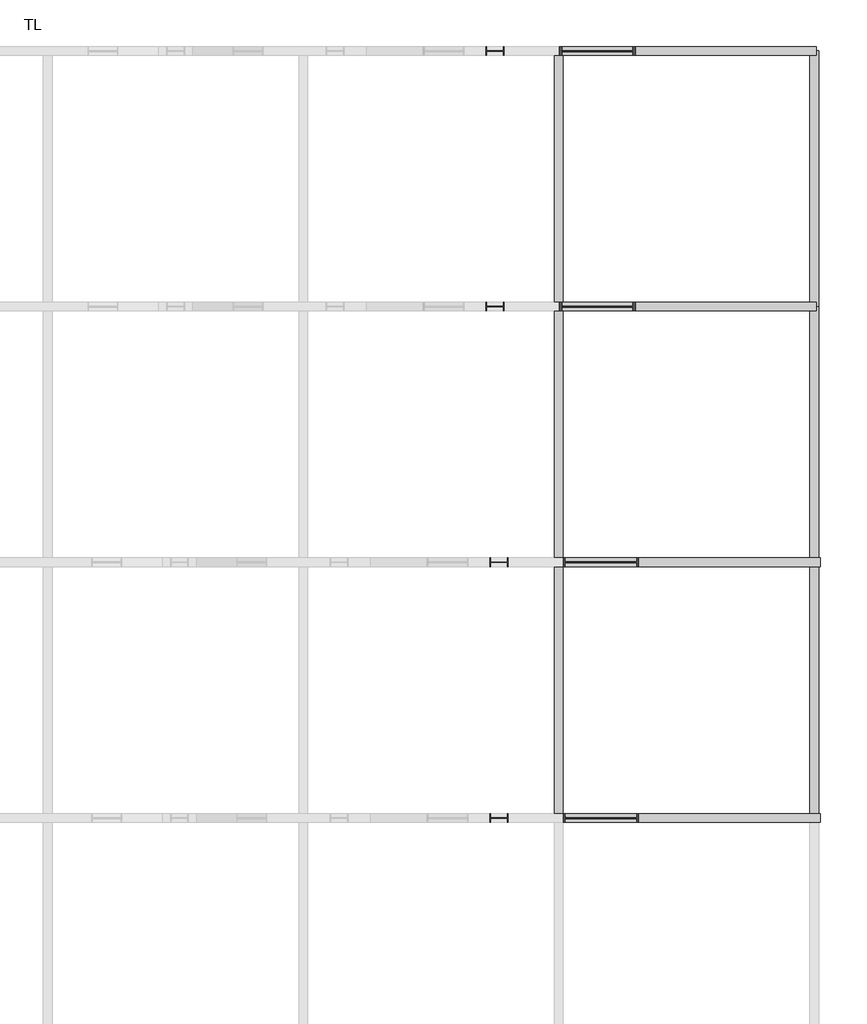
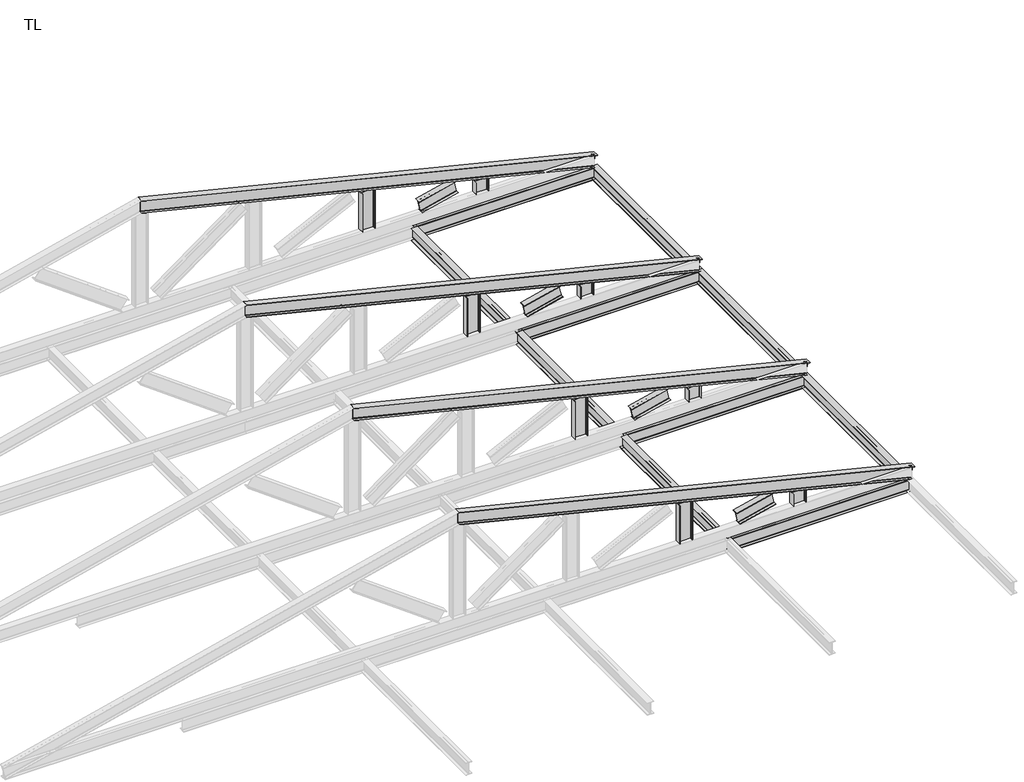
# One storey, part 4 of 4: 26 beams.
"""IFC4 building model written with IfcOpenShell, lengths in millimetres."""

from ifc_helpers import new_model, si_unit, frame, origin, place, context, project, spatial, polyline, circle_curve, ellipse_curve, transform, mapped, element, save
from ifc_brep_helpers import plane_surface, revolved_surface, advanced_brep
from components import w_shapes_w14x30_920474df, w_shapes_w14x30_b44ec7f2, w_shapes_w14x30_809da129, w_shapes_w14x30_95bb247d

model = new_model("IFC4")

# Units and contexts
model_context = context("Model", 3, world=origin())
ifc_project = project(units=[si_unit("LENGTHUNIT", "METRE", prefix="MILLI")], contexts=[model_context])

# Site, building, storey
site = spatial("IfcSite", under=ifc_project)
building = spatial("IfcBuilding", under=site)
storey = spatial("IfcBuildingStorey", under=building, Name="TL", Elevation=8534.4)

# Beams
placement = place(None, origin())
element("IfcBeam", 1, ObjectType="W Shapes : W14X30", at=placement, inside=storey, context=model_context, shape_type="AdvancedBrep", body=[
    advanced_brep(
    [(6535.1598435, 14124.3335479, 8538.7295322), (6535.1598435, 14052.4515479, 8538.7295322), (6537.5667365, 14042.2915479, 8548.6003207), (6611.1574921, 14042.2915479, 8850.3996793), (6613.5643852, 14052.4515479, 8860.2704678), (6613.5643852, 14124.3335479, 8860.2704678), (6615.8810198, 14124.3335479, 8869.7711017), (6615.8810198, 13953.3915479, 8869.7711017), (6613.5643852, 13953.3915479, 8860.2704678), (6613.5643852, 14025.2735479, 8860.2704678), (6611.1574921, 14035.4335479, 8850.3996793), (6537.5667365, 14035.4335479, 8548.6003207), (6535.1598435, 14025.2735479, 8538.7295322), (6535.1598435, 13953.3915479, 8538.7295322), (6532.8432089, 13953.3915479, 8529.2288983), (6532.8432089, 14124.3335479, 8529.2288983), (-5925.6378857, 14124.3335479, 11577.1704505), (-5925.6378857, 14052.4515479, 11577.1704505), (-5925.6378857, 14042.2915479, 11587.6281358), (-5925.6378857, 14042.2915479, 11907.3718642), (-5925.6378857, 14052.4515479, 11917.8295495), (-5925.6378857, 14124.3335479, 11917.8295495), (-5925.6378857, 14124.3335479, 11927.8950717), (-5925.6378857, 13953.3915479, 11927.8950717), (-5925.6378857, 13953.3915479, 11917.8295495), (-5925.6378857, 14025.2735479, 11917.8295495), (-5925.6378857, 14035.4335479, 11907.3718642), (-5925.6378857, 14035.4335479, 11587.6281358), (-5925.6378857, 14025.2735479, 11577.1704505), (-5925.6378857, 13953.3915479, 11577.1704505), (-5925.6378857, 13953.3915479, 11567.1049283), (-5925.6378857, 14124.3335479, 11567.1049283)],
    [
        (0, 1),
        (1, 2, circle_curve(frame((6537.5667365, 14052.4515479, 8548.6003207), z_axis=(-0.971534301878756, 0.0, 0.23689892417011588), x_axis=(0.0, -1.0, 0.0)), 10.16)),
        (2, 3),
        (3, 4, circle_curve(frame((6611.1574921, 14052.4515479, 8850.3996793), z_axis=(-0.971534301878756, 0.0, 0.23689892417011588), x_axis=(0.23689892417011588, 0.0, 0.971534301878756)), 10.16)),
        (4, 5),
        (5, 6),
        (6, 7),
        (7, 8),
        (8, 9),
        (9, 10, circle_curve(frame((6611.1574921, 14025.2735479, 8850.3996793), z_axis=(-0.971534301878756, 0.0, 0.23689892417011588), x_axis=(0.0, 1.0, 0.0)), 10.16)),
        (10, 11),
        (11, 12, circle_curve(frame((6537.5667365, 14025.2735479, 8548.6003207), z_axis=(-0.971534301878756, 0.0, 0.23689892417011588), x_axis=(-0.23689892417011588, 0.0, -0.971534301878756)), 10.16)),
        (12, 13),
        (13, 14),
        (14, 15),
        (15, 0),
        (0, 16),
        (16, 17),
        (17, 1),
        (17, 18, ellipse_curve(frame((-5925.6378857, 14052.4515479, 11587.6281358), z_axis=(-1.0, 0.0, 0.0), x_axis=(0.0, 0.0, 1.0)), 10.4576853, 10.16)),
        (18, 2),
        (18, 19),
        (19, 3),
        (19, 20, ellipse_curve(frame((-5925.6378857, 14052.4515479, 11907.3718642), z_axis=(-1.0, 0.0, 0.0), x_axis=(0.0, 0.0, 1.0)), 10.4576853, 10.16)),
        (20, 4),
        (20, 21),
        (21, 5),
        (21, 22),
        (22, 6),
        (22, 23),
        (23, 7),
        (23, 24),
        (24, 8),
        (24, 25),
        (25, 9),
        (25, 26, ellipse_curve(frame((-5925.6378857, 14025.2735479, 11907.3718642), z_axis=(-1.0, 0.0, 0.0), x_axis=(0.0, 0.0, 1.0)), 10.4576853, 10.16)),
        (26, 10),
        (26, 27),
        (27, 11),
        (27, 28, ellipse_curve(frame((-5925.6378857, 14025.2735479, 11587.6281358), z_axis=(-1.0, 0.0, 0.0), x_axis=(0.0, 0.0, 1.0)), 10.4576853, 10.16)),
        (28, 12),
        (28, 29),
        (29, 13),
        (29, 30),
        (30, 14),
        (30, 31),
        (31, 15),
        (31, 16),
    ],
    [
        plane_surface(frame((6574.3621143, 14038.8625479, 8699.5), z_axis=(0.971534301878756, 0.0, -0.23689892417011588), x_axis=(0.23689892417011588, 0.0, 0.971534301878756))),
        plane_surface(frame((6535.1598435, 14088.3925479, 8538.7295322), z_axis=(0.23689892417011588, 0.0, 0.971534301878756), x_axis=(0.0, -1.0, 0.0))),
        revolved_surface(polyline([(-5928.044778771774, 14042.2915479, 11588.215032583868), (6537.566736564032, 14042.2915479, 8548.600320684385)]), (6537.5667365, 14052.4515479, 8548.6003207), (-0.971534301878756, 0.0, 0.23689892417011588)),
        plane_surface(frame((6574.3621143, 14042.2915479, 8699.5), z_axis=(0.0, 1.0, 0.0), x_axis=(0.23689892417011588, 0.0, 0.971534301878756))),
        revolved_surface(polyline([(-5925.637885691734, 14052.4515479, 11917.82954953391), (6613.564385199924, 14052.4515479, 8860.270467799688)]), (6611.1574921, 14052.4515479, 8850.3996793), (-0.971534301878756, 0.0, 0.23689892417011588)),
        plane_surface(frame((6613.5643852, 14088.3925479, 8860.2704678), z_axis=(-0.23689892417011588, 0.0, -0.971534301878756), x_axis=(0.0, 1.0, 0.0))),
        plane_surface(frame((6614.7227025, 14124.3335479, 8865.0207848), z_axis=(0.0, 1.0, 0.0), x_axis=(0.23689892417011588, 0.0, 0.971534301878756))),
        plane_surface(frame((6615.8810198, 14038.8625479, 8869.7711017), z_axis=(0.23689892417011588, 0.0, 0.971534301878756), x_axis=(0.0, -1.0, 0.0))),
        plane_surface(frame((6614.7227025, 13953.3915479, 8865.0207848), z_axis=(0.0, -1.0, 0.0), x_axis=(-0.23689892417011588, 0.0, -0.971534301878756))),
        plane_surface(frame((6613.5643852, 13989.3325479, 8860.2704678), z_axis=(-0.23689892417011588, 0.0, -0.971534301878756), x_axis=(0.0, 1.0, 0.0))),
        revolved_surface(polyline([(-5928.044778761302, 14035.4335479, 11907.95876102682), (6611.157492130355, 14035.4335479, 8850.3996792926)]), (6611.1574921, 14025.2735479, 8850.3996793), (-0.971534301878756, 0.0, 0.23689892417011588)),
        plane_surface(frame((6574.3621143, 14035.4335479, 8699.5), z_axis=(0.0, -1.0, 0.0), x_axis=(-0.23689892417011588, 0.0, -0.971534301878756))),
        revolved_surface(polyline([(-5930.451671841342, 14025.2735479, 11578.34424407678), (6535.1598434944635, 14025.2735479, 8538.729532177296)]), (6537.5667365, 14025.2735479, 8548.6003207), (-0.971534301878756, 0.0, 0.23689892417011588)),
        plane_surface(frame((6535.1598435, 13989.3325479, 8538.7295322), z_axis=(0.23689892417011588, 0.0, 0.971534301878756), x_axis=(0.0, -1.0, 0.0))),
        plane_surface(frame((6534.0015262, 13953.3915479, 8533.9792152), z_axis=(0.0, -1.0, 0.0), x_axis=(-0.23689892417011588, 0.0, -0.971534301878756))),
        plane_surface(frame((6532.8432089, 14038.8625479, 8529.2288983), z_axis=(-0.23689892417011588, 0.0, -0.971534301878756), x_axis=(0.0, 1.0, 0.0))),
        plane_surface(frame((6534.0015262, 14124.3335479, 8533.9792152), z_axis=(0.0, 1.0, 0.0), x_axis=(0.23689892417011588, 0.0, 0.971534301878756))),
        plane_surface(frame((-5925.6378857, 14038.8625479, 11927.8950717), z_axis=(-1.0, 0.0, 0.0), x_axis=(0.0, 1.0, 0.0))),
    ],
    [
        (0, [[1, 2, 3, 4, 5, 6, 7, 8, 9, 10, 11, 12, 13, 14, 15, 16]]),
        (1, [[-1, 17, 18, 19]]),
        (2, [[-2, -19, 20, 21]]),
        (3, [[-3, -21, 22, 23]]),
        (4, [[-4, -23, 24, 25]]),
        (5, [[-5, -25, 26, 27]]),
        (6, [[-6, -27, 28, 29]]),
        (7, [[-7, -29, 30, 31]]),
        (8, [[-8, -31, 32, 33]]),
        (9, [[-9, -33, 34, 35]]),
        (10, [[-10, -35, 36, 37]]),
        (11, [[-11, -37, 38, 39]]),
        (12, [[-12, -39, 40, 41]]),
        (13, [[-13, -41, 42, 43]]),
        (14, [[-14, -43, 44, 45]]),
        (15, [[-15, -45, 46, 47]]),
        (16, [[-16, -47, 48, -17]]),
        (17, [[-48, -46, -44, -42, -40, -38, -36, -34, -32, -30, -28, -26, -24, -22, -20, -18]]),
    ],
),
])
element("IfcBeam", 2, ObjectType="W Shapes : W14X30", at=placement, inside=storey, context=model_context, shape_type="AdvancedBrep", body=[
    advanced_brep(
    [(6611.3598435, 9124.3335479, 8538.7295322), (6611.3598435, 9052.4515479, 8538.7295322), (6613.7667365, 9042.2915479, 8548.6003207), (6687.3574921, 9042.2915479, 8850.3996793), (6689.7643852, 9052.4515479, 8860.2704678), (6689.7643852, 9124.3335479, 8860.2704678), (6692.0810198, 9124.3335479, 8869.7711017), (6692.0810198, 8953.3915479, 8869.7711017), (6689.7643852, 8953.3915479, 8860.2704678), (6689.7643852, 9025.2735479, 8860.2704678), (6687.3574921, 9035.4335479, 8850.3996793), (6613.7667365, 9035.4335479, 8548.6003207), (6611.3598435, 9025.2735479, 8538.7295322), (6611.3598435, 8953.3915479, 8538.7295322), (6609.0432089, 8953.3915479, 8529.2288983), (6609.0432089, 9124.3335479, 8529.2288983), (-5849.4378857, 9124.3335479, 11577.1704505), (-5849.4378857, 9052.4515479, 11577.1704505), (-5849.4378857, 9042.2915479, 11587.6281358), (-5849.4378857, 9042.2915479, 11907.3718642), (-5849.4378857, 9052.4515479, 11917.8295495), (-5849.4378857, 9124.3335479, 11917.8295495), (-5849.4378857, 9124.3335479, 11927.8950717), (-5849.4378857, 8953.3915479, 11927.8950717), (-5849.4378857, 8953.3915479, 11917.8295495), (-5849.4378857, 9025.2735479, 11917.8295495), (-5849.4378857, 9035.4335479, 11907.3718642), (-5849.4378857, 9035.4335479, 11587.6281358), (-5849.4378857, 9025.2735479, 11577.1704505), (-5849.4378857, 8953.3915479, 11577.1704505), (-5849.4378857, 8953.3915479, 11567.1049283), (-5849.4378857, 9124.3335479, 11567.1049283)],
    [
        (0, 1),
        (1, 2, circle_curve(frame((6613.7667365, 9052.4515479, 8548.6003207), z_axis=(-0.971534301878756, 0.0, 0.23689892417011588), x_axis=(0.0, -1.0, 0.0)), 10.16)),
        (2, 3),
        (3, 4, circle_curve(frame((6687.3574921, 9052.4515479, 8850.3996793), z_axis=(-0.971534301878756, 0.0, 0.23689892417011588), x_axis=(0.23689892417011588, 0.0, 0.971534301878756)), 10.16)),
        (4, 5),
        (5, 6),
        (6, 7),
        (7, 8),
        (8, 9),
        (9, 10, circle_curve(frame((6687.3574921, 9025.2735479, 8850.3996793), z_axis=(-0.971534301878756, 0.0, 0.23689892417011588), x_axis=(0.0, 1.0, 0.0)), 10.16)),
        (10, 11),
        (11, 12, circle_curve(frame((6613.7667365, 9025.2735479, 8548.6003207), z_axis=(-0.971534301878756, 0.0, 0.23689892417011588), x_axis=(-0.23689892417011588, 0.0, -0.971534301878756)), 10.16)),
        (12, 13),
        (13, 14),
        (14, 15),
        (15, 0),
        (0, 16),
        (16, 17),
        (17, 1),
        (17, 18, ellipse_curve(frame((-5849.4378857, 9052.4515479, 11587.6281358), z_axis=(-1.0, 0.0, 0.0), x_axis=(0.0, 0.0, 1.0)), 10.4576853, 10.16)),
        (18, 2),
        (18, 19),
        (19, 3),
        (19, 20, ellipse_curve(frame((-5849.4378857, 9052.4515479, 11907.3718642), z_axis=(-1.0, 0.0, 0.0), x_axis=(0.0, 0.0, 1.0)), 10.4576853, 10.16)),
        (20, 4),
        (20, 21),
        (21, 5),
        (21, 22),
        (22, 6),
        (22, 23),
        (23, 7),
        (23, 24),
        (24, 8),
        (24, 25),
        (25, 9),
        (25, 26, ellipse_curve(frame((-5849.4378857, 9025.2735479, 11907.3718642), z_axis=(-1.0, 0.0, 0.0), x_axis=(0.0, 0.0, 1.0)), 10.4576853, 10.16)),
        (26, 10),
        (26, 27),
        (27, 11),
        (27, 28, ellipse_curve(frame((-5849.4378857, 9025.2735479, 11587.6281358), z_axis=(-1.0, 0.0, 0.0), x_axis=(0.0, 0.0, 1.0)), 10.4576853, 10.16)),
        (28, 12),
        (28, 29),
        (29, 13),
        (29, 30),
        (30, 14),
        (30, 31),
        (31, 15),
        (31, 16),
    ],
    [
        plane_surface(frame((6650.5621143, 9038.8625479, 8699.5), z_axis=(0.971534301878756, 0.0, -0.23689892417011588), x_axis=(0.23689892417011588, 0.0, 0.971534301878756))),
        plane_surface(frame((6611.3598435, 9088.3925479, 8538.7295322), z_axis=(0.23689892417011588, 0.0, 0.971534301878756), x_axis=(0.0, -1.0, 0.0))),
        revolved_surface(polyline([(-5851.844778771774, 9042.2915479, 11588.215032583868), (6613.766736564033, 9042.2915479, 8548.600320684385)]), (6613.7667365, 9052.4515479, 8548.6003207), (-0.971534301878756, 0.0, 0.23689892417011588)),
        plane_surface(frame((6650.5621143, 9042.2915479, 8699.5), z_axis=(0.0, 1.0, 0.0), x_axis=(0.23689892417011588, 0.0, 0.971534301878756))),
        revolved_surface(polyline([(-5849.437885691734, 9052.4515479, 11917.82954953391), (6689.764385199924, 9052.4515479, 8860.270467799688)]), (6687.3574921, 9052.4515479, 8850.3996793), (-0.971534301878756, 0.0, 0.23689892417011588)),
        plane_surface(frame((6689.7643852, 9088.3925479, 8860.2704678), z_axis=(-0.23689892417011588, 0.0, -0.971534301878756), x_axis=(0.0, 1.0, 0.0))),
        plane_surface(frame((6690.9227025, 9124.3335479, 8865.0207848), z_axis=(0.0, 1.0, 0.0), x_axis=(0.23689892417011588, 0.0, 0.971534301878756))),
        plane_surface(frame((6692.0810198, 9038.8625479, 8869.7711017), z_axis=(0.23689892417011588, 0.0, 0.971534301878756), x_axis=(0.0, -1.0, 0.0))),
        plane_surface(frame((6690.9227025, 8953.3915479, 8865.0207848), z_axis=(0.0, -1.0, 0.0), x_axis=(-0.23689892417011588, 0.0, -0.971534301878756))),
        plane_surface(frame((6689.7643852, 8989.3325479, 8860.2704678), z_axis=(-0.23689892417011588, 0.0, -0.971534301878756), x_axis=(0.0, 1.0, 0.0))),
        revolved_surface(polyline([(-5851.844778761302, 9035.4335479, 11907.95876102682), (6687.357492130355, 9035.4335479, 8850.3996792926)]), (6687.3574921, 9025.2735479, 8850.3996793), (-0.971534301878756, 0.0, 0.23689892417011588)),
        plane_surface(frame((6650.5621143, 9035.4335479, 8699.5), z_axis=(0.0, -1.0, 0.0), x_axis=(-0.23689892417011588, 0.0, -0.971534301878756))),
        revolved_surface(polyline([(-5854.251671841343, 9025.2735479, 11578.34424407678), (6611.359843494464, 9025.2735479, 8538.729532177296)]), (6613.7667365, 9025.2735479, 8548.6003207), (-0.971534301878756, 0.0, 0.23689892417011588)),
        plane_surface(frame((6611.3598435, 8989.3325479, 8538.7295322), z_axis=(0.23689892417011588, 0.0, 0.971534301878756), x_axis=(0.0, -1.0, 0.0))),
        plane_surface(frame((6610.2015262, 8953.3915479, 8533.9792152), z_axis=(0.0, -1.0, 0.0), x_axis=(-0.23689892417011588, 0.0, -0.971534301878756))),
        plane_surface(frame((6609.0432089, 9038.8625479, 8529.2288983), z_axis=(-0.23689892417011588, 0.0, -0.971534301878756), x_axis=(0.0, 1.0, 0.0))),
        plane_surface(frame((6610.2015262, 9124.3335479, 8533.9792152), z_axis=(0.0, 1.0, 0.0), x_axis=(0.23689892417011588, 0.0, 0.971534301878756))),
        plane_surface(frame((-5849.4378857, 9038.8625479, 11927.8950717), z_axis=(-1.0, 0.0, 0.0), x_axis=(0.0, 1.0, 0.0))),
    ],
    [
        (0, [[1, 2, 3, 4, 5, 6, 7, 8, 9, 10, 11, 12, 13, 14, 15, 16]]),
        (1, [[-1, 17, 18, 19]]),
        (2, [[-2, -19, 20, 21]]),
        (3, [[-3, -21, 22, 23]]),
        (4, [[-4, -23, 24, 25]]),
        (5, [[-5, -25, 26, 27]]),
        (6, [[-6, -27, 28, 29]]),
        (7, [[-7, -29, 30, 31]]),
        (8, [[-8, -31, 32, 33]]),
        (9, [[-9, -33, 34, 35]]),
        (10, [[-10, -35, 36, 37]]),
        (11, [[-11, -37, 38, 39]]),
        (12, [[-12, -39, 40, 41]]),
        (13, [[-13, -41, 42, 43]]),
        (14, [[-14, -43, 44, 45]]),
        (15, [[-15, -45, 46, 47]]),
        (16, [[-16, -47, 48, -17]]),
        (17, [[-48, -46, -44, -42, -40, -38, -36, -34, -32, -30, -28, -26, -24, -22, -20, -18]]),
    ],
),
])
element("IfcBeam", 3, ObjectType="W Shapes : W14X30", at=placement, inside=storey, context=model_context, shape_type="AdvancedBrep", body=[
    advanced_brep(
    [(6611.3598435, 4124.3335479, 8538.7295322), (6611.3598435, 4052.4515479, 8538.7295322), (6613.7667365, 4042.2915479, 8548.6003207), (6687.3574921, 4042.2915479, 8850.3996793), (6689.7643852, 4052.4515479, 8860.2704678), (6689.7643852, 4124.3335479, 8860.2704678), (6692.0810198, 4124.3335479, 8869.7711017), (6692.0810198, 3953.3915479, 8869.7711017), (6689.7643852, 3953.3915479, 8860.2704678), (6689.7643852, 4025.2735479, 8860.2704678), (6687.3574921, 4035.4335479, 8850.3996793), (6613.7667365, 4035.4335479, 8548.6003207), (6611.3598435, 4025.2735479, 8538.7295322), (6611.3598435, 3953.3915479, 8538.7295322), (6609.0432089, 3953.3915479, 8529.2288983), (6609.0432089, 4124.3335479, 8529.2288983), (-5849.4378857, 4124.3335479, 11577.1704505), (-5849.4378857, 4052.4515479, 11577.1704505), (-5849.4378857, 4042.2915479, 11587.6281358), (-5849.4378857, 4042.2915479, 11907.3718642), (-5849.4378857, 4052.4515479, 11917.8295495), (-5849.4378857, 4124.3335479, 11917.8295495), (-5849.4378857, 4124.3335479, 11927.8950717), (-5849.4378857, 3953.3915479, 11927.8950717), (-5849.4378857, 3953.3915479, 11917.8295495), (-5849.4378857, 4025.2735479, 11917.8295495), (-5849.4378857, 4035.4335479, 11907.3718642), (-5849.4378857, 4035.4335479, 11587.6281358), (-5849.4378857, 4025.2735479, 11577.1704505), (-5849.4378857, 3953.3915479, 11577.1704505), (-5849.4378857, 3953.3915479, 11567.1049283), (-5849.4378857, 4124.3335479, 11567.1049283)],
    [
        (0, 1),
        (1, 2, circle_curve(frame((6613.7667365, 4052.4515479, 8548.6003207), z_axis=(-0.971534301878756, 0.0, 0.23689892417011588), x_axis=(0.0, -1.0, 0.0)), 10.16)),
        (2, 3),
        (3, 4, circle_curve(frame((6687.3574921, 4052.4515479, 8850.3996793), z_axis=(-0.971534301878756, 0.0, 0.23689892417011588), x_axis=(0.23689892417011588, 0.0, 0.971534301878756)), 10.16)),
        (4, 5),
        (5, 6),
        (6, 7),
        (7, 8),
        (8, 9),
        (9, 10, circle_curve(frame((6687.3574921, 4025.2735479, 8850.3996793), z_axis=(-0.971534301878756, 0.0, 0.23689892417011588), x_axis=(0.0, 1.0, 0.0)), 10.16)),
        (10, 11),
        (11, 12, circle_curve(frame((6613.7667365, 4025.2735479, 8548.6003207), z_axis=(-0.971534301878756, 0.0, 0.23689892417011588), x_axis=(-0.23689892417011588, 0.0, -0.971534301878756)), 10.16)),
        (12, 13),
        (13, 14),
        (14, 15),
        (15, 0),
        (0, 16),
        (16, 17),
        (17, 1),
        (17, 18, ellipse_curve(frame((-5849.4378857, 4052.4515479, 11587.6281358), z_axis=(-1.0, 0.0, 0.0), x_axis=(0.0, 0.0, 1.0)), 10.4576853, 10.16)),
        (18, 2),
        (18, 19),
        (19, 3),
        (19, 20, ellipse_curve(frame((-5849.4378857, 4052.4515479, 11907.3718642), z_axis=(-1.0, 0.0, 0.0), x_axis=(0.0, 0.0, 1.0)), 10.4576853, 10.16)),
        (20, 4),
        (20, 21),
        (21, 5),
        (21, 22),
        (22, 6),
        (22, 23),
        (23, 7),
        (23, 24),
        (24, 8),
        (24, 25),
        (25, 9),
        (25, 26, ellipse_curve(frame((-5849.4378857, 4025.2735479, 11907.3718642), z_axis=(-1.0, 0.0, 0.0), x_axis=(0.0, 0.0, 1.0)), 10.4576853, 10.16)),
        (26, 10),
        (26, 27),
        (27, 11),
        (27, 28, ellipse_curve(frame((-5849.4378857, 4025.2735479, 11587.6281358), z_axis=(-1.0, 0.0, 0.0), x_axis=(0.0, 0.0, 1.0)), 10.4576853, 10.16)),
        (28, 12),
        (28, 29),
        (29, 13),
        (29, 30),
        (30, 14),
        (30, 31),
        (31, 15),
        (31, 16),
    ],
    [
        plane_surface(frame((6650.5621143, 4038.8625479, 8699.5), z_axis=(0.971534301878756, 0.0, -0.23689892417011588), x_axis=(0.23689892417011588, 0.0, 0.971534301878756))),
        plane_surface(frame((6611.3598435, 4088.3925479, 8538.7295322), z_axis=(0.23689892417011588, 0.0, 0.971534301878756), x_axis=(0.0, -1.0, 0.0))),
        revolved_surface(polyline([(-5851.844778771774, 4042.2915479000003, 11588.215032583868), (6613.766736564033, 4042.2915479000003, 8548.600320684385)]), (6613.7667365, 4052.4515479, 8548.6003207), (-0.971534301878756, 0.0, 0.23689892417011588)),
        plane_surface(frame((6650.5621143, 4042.2915479, 8699.5), z_axis=(0.0, 1.0, 0.0), x_axis=(0.23689892417011588, 0.0, 0.971534301878756))),
        revolved_surface(polyline([(-5849.437885691734, 4052.4515479, 11917.82954953391), (6689.764385199924, 4052.4515479, 8860.270467799688)]), (6687.3574921, 4052.4515479, 8850.3996793), (-0.971534301878756, 0.0, 0.23689892417011588)),
        plane_surface(frame((6689.7643852, 4088.3925479, 8860.2704678), z_axis=(-0.23689892417011588, 0.0, -0.971534301878756), x_axis=(0.0, 1.0, 0.0))),
        plane_surface(frame((6690.9227025, 4124.3335479, 8865.0207848), z_axis=(0.0, 1.0, 0.0), x_axis=(0.23689892417011588, 0.0, 0.971534301878756))),
        plane_surface(frame((6692.0810198, 4038.8625479, 8869.7711017), z_axis=(0.23689892417011588, 0.0, 0.971534301878756), x_axis=(0.0, -1.0, 0.0))),
        plane_surface(frame((6690.9227025, 3953.3915479, 8865.0207848), z_axis=(0.0, -1.0, 0.0), x_axis=(-0.23689892417011588, 0.0, -0.971534301878756))),
        plane_surface(frame((6689.7643852, 3989.3325479, 8860.2704678), z_axis=(-0.23689892417011588, 0.0, -0.971534301878756), x_axis=(0.0, 1.0, 0.0))),
        revolved_surface(polyline([(-5851.844778761302, 4035.4335478999997, 11907.95876102682), (6687.357492130355, 4035.4335478999997, 8850.3996792926)]), (6687.3574921, 4025.2735479, 8850.3996793), (-0.971534301878756, 0.0, 0.23689892417011588)),
        plane_surface(frame((6650.5621143, 4035.4335479, 8699.5), z_axis=(0.0, -1.0, 0.0), x_axis=(-0.23689892417011588, 0.0, -0.971534301878756))),
        revolved_surface(polyline([(-5854.251671841343, 4025.2735479, 11578.34424407678), (6611.359843494464, 4025.2735479, 8538.729532177296)]), (6613.7667365, 4025.2735479, 8548.6003207), (-0.971534301878756, 0.0, 0.23689892417011588)),
        plane_surface(frame((6611.3598435, 3989.3325479, 8538.7295322), z_axis=(0.23689892417011588, 0.0, 0.971534301878756), x_axis=(0.0, -1.0, 0.0))),
        plane_surface(frame((6610.2015262, 3953.3915479, 8533.9792152), z_axis=(0.0, -1.0, 0.0), x_axis=(-0.23689892417011588, 0.0, -0.971534301878756))),
        plane_surface(frame((6609.0432089, 4038.8625479, 8529.2288983), z_axis=(-0.23689892417011588, 0.0, -0.971534301878756), x_axis=(0.0, 1.0, 0.0))),
        plane_surface(frame((6610.2015262, 4124.3335479, 8533.9792152), z_axis=(0.0, 1.0, 0.0), x_axis=(0.23689892417011588, 0.0, 0.971534301878756))),
        plane_surface(frame((-5849.4378857, 4038.8625479, 11927.8950717), z_axis=(-1.0, 0.0, 0.0), x_axis=(0.0, 1.0, 0.0))),
    ],
    [
        (0, [[1, 2, 3, 4, 5, 6, 7, 8, 9, 10, 11, 12, 13, 14, 15, 16]]),
        (1, [[-1, 17, 18, 19]]),
        (2, [[-2, -19, 20, 21]]),
        (3, [[-3, -21, 22, 23]]),
        (4, [[-4, -23, 24, 25]]),
        (5, [[-5, -25, 26, 27]]),
        (6, [[-6, -27, 28, 29]]),
        (7, [[-7, -29, 30, 31]]),
        (8, [[-8, -31, 32, 33]]),
        (9, [[-9, -33, 34, 35]]),
        (10, [[-10, -35, 36, 37]]),
        (11, [[-11, -37, 38, 39]]),
        (12, [[-12, -39, 40, 41]]),
        (13, [[-13, -41, 42, 43]]),
        (14, [[-14, -43, 44, 45]]),
        (15, [[-15, -45, 46, 47]]),
        (16, [[-16, -47, 48, -17]]),
        (17, [[-48, -46, -44, -42, -40, -38, -36, -34, -32, -30, -28, -26, -24, -22, -20, -18]]),
    ],
),
])
element("IfcBeam", 4, ObjectType="W Shapes : W14X30", at=placement, inside=storey, context=model_context, shape_type="AdvancedBrep", body=[
    advanced_brep(
    [(6535.1598435, 19124.3335479, 8538.7295322), (6535.1598435, 19052.4515479, 8538.7295322), (6537.5667365, 19042.2915479, 8548.6003207), (6611.1574921, 19042.2915479, 8850.3996793), (6613.5643852, 19052.4515479, 8860.2704678), (6613.5643852, 19124.3335479, 8860.2704678), (6615.8810198, 19124.3335479, 8869.7711017), (6615.8810198, 18953.3915479, 8869.7711017), (6613.5643852, 18953.3915479, 8860.2704678), (6613.5643852, 19025.2735479, 8860.2704678), (6611.1574921, 19035.4335479, 8850.3996793), (6537.5667365, 19035.4335479, 8548.6003207), (6535.1598435, 19025.2735479, 8538.7295322), (6535.1598435, 18953.3915479, 8538.7295322), (6532.8432089, 18953.3915479, 8529.2288983), (6532.8432089, 19124.3335479, 8529.2288983), (-5925.6378857, 19124.3335479, 11577.1704505), (-5925.6378857, 19052.4515479, 11577.1704505), (-5925.6378857, 19042.2915479, 11587.6281358), (-5925.6378857, 19042.2915479, 11907.3718642), (-5925.6378857, 19052.4515479, 11917.8295495), (-5925.6378857, 19124.3335479, 11917.8295495), (-5925.6378857, 19124.3335479, 11927.8950717), (-5925.6378857, 18953.3915479, 11927.8950717), (-5925.6378857, 18953.3915479, 11917.8295495), (-5925.6378857, 19025.2735479, 11917.8295495), (-5925.6378857, 19035.4335479, 11907.3718642), (-5925.6378857, 19035.4335479, 11587.6281358), (-5925.6378857, 19025.2735479, 11577.1704505), (-5925.6378857, 18953.3915479, 11577.1704505), (-5925.6378857, 18953.3915479, 11567.1049283), (-5925.6378857, 19124.3335479, 11567.1049283)],
    [
        (0, 1),
        (1, 2, circle_curve(frame((6537.5667365, 19052.4515479, 8548.6003207), z_axis=(-0.971534301878756, 0.0, 0.23689892417011588), x_axis=(0.0, -1.0, 0.0)), 10.16)),
        (2, 3),
        (3, 4, circle_curve(frame((6611.1574921, 19052.4515479, 8850.3996793), z_axis=(-0.971534301878756, 0.0, 0.23689892417011588), x_axis=(0.23689892417011588, 0.0, 0.971534301878756)), 10.16)),
        (4, 5),
        (5, 6),
        (6, 7),
        (7, 8),
        (8, 9),
        (9, 10, circle_curve(frame((6611.1574921, 19025.2735479, 8850.3996793), z_axis=(-0.971534301878756, 0.0, 0.23689892417011588), x_axis=(0.0, 1.0, 0.0)), 10.16)),
        (10, 11),
        (11, 12, circle_curve(frame((6537.5667365, 19025.2735479, 8548.6003207), z_axis=(-0.971534301878756, 0.0, 0.23689892417011588), x_axis=(-0.23689892417011588, 0.0, -0.971534301878756)), 10.16)),
        (12, 13),
        (13, 14),
        (14, 15),
        (15, 0),
        (0, 16),
        (16, 17),
        (17, 1),
        (17, 18, ellipse_curve(frame((-5925.6378857, 19052.4515479, 11587.6281358), z_axis=(-1.0, 0.0, 0.0), x_axis=(0.0, 0.0, 1.0)), 10.4576853, 10.16)),
        (18, 2),
        (18, 19),
        (19, 3),
        (19, 20, ellipse_curve(frame((-5925.6378857, 19052.4515479, 11907.3718642), z_axis=(-1.0, 0.0, 0.0), x_axis=(0.0, 0.0, 1.0)), 10.4576853, 10.16)),
        (20, 4),
        (20, 21),
        (21, 5),
        (21, 22),
        (22, 6),
        (22, 23),
        (23, 7),
        (23, 24),
        (24, 8),
        (24, 25),
        (25, 9),
        (25, 26, ellipse_curve(frame((-5925.6378857, 19025.2735479, 11907.3718642), z_axis=(-1.0, 0.0, 0.0), x_axis=(0.0, 0.0, 1.0)), 10.4576853, 10.16)),
        (26, 10),
        (26, 27),
        (27, 11),
        (27, 28, ellipse_curve(frame((-5925.6378857, 19025.2735479, 11587.6281358), z_axis=(-1.0, 0.0, 0.0), x_axis=(0.0, 0.0, 1.0)), 10.4576853, 10.16)),
        (28, 12),
        (28, 29),
        (29, 13),
        (29, 30),
        (30, 14),
        (30, 31),
        (31, 15),
        (31, 16),
    ],
    [
        plane_surface(frame((6574.3621143, 19038.8625479, 8699.5), z_axis=(0.971534301878756, 0.0, -0.23689892417011588), x_axis=(0.23689892417011588, 0.0, 0.971534301878756))),
        plane_surface(frame((6535.1598435, 19088.3925479, 8538.7295322), z_axis=(0.23689892417011588, 0.0, 0.971534301878756), x_axis=(0.0, -1.0, 0.0))),
        revolved_surface(polyline([(-5928.044778771774, 19042.2915479, 11588.215032583868), (6537.566736564032, 19042.2915479, 8548.600320684385)]), (6537.5667365, 19052.4515479, 8548.6003207), (-0.971534301878756, 0.0, 0.23689892417011588)),
        plane_surface(frame((6574.3621143, 19042.2915479, 8699.5), z_axis=(0.0, 1.0, 0.0), x_axis=(0.23689892417011588, 0.0, 0.971534301878756))),
        revolved_surface(polyline([(-5925.637885691734, 19052.4515479, 11917.82954953391), (6613.564385199924, 19052.4515479, 8860.270467799688)]), (6611.1574921, 19052.4515479, 8850.3996793), (-0.971534301878756, 0.0, 0.23689892417011588)),
        plane_surface(frame((6613.5643852, 19088.3925479, 8860.2704678), z_axis=(-0.23689892417011588, 0.0, -0.971534301878756), x_axis=(0.0, 1.0, 0.0))),
        plane_surface(frame((6614.7227025, 19124.3335479, 8865.0207848), z_axis=(0.0, 1.0, 0.0), x_axis=(0.23689892417011588, 0.0, 0.971534301878756))),
        plane_surface(frame((6615.8810198, 19038.8625479, 8869.7711017), z_axis=(0.23689892417011588, 0.0, 0.971534301878756), x_axis=(0.0, -1.0, 0.0))),
        plane_surface(frame((6614.7227025, 18953.3915479, 8865.0207848), z_axis=(0.0, -1.0, 0.0), x_axis=(-0.23689892417011588, 0.0, -0.971534301878756))),
        plane_surface(frame((6613.5643852, 18989.3325479, 8860.2704678), z_axis=(-0.23689892417011588, 0.0, -0.971534301878756), x_axis=(0.0, 1.0, 0.0))),
        revolved_surface(polyline([(-5928.044778761302, 19035.4335479, 11907.95876102682), (6611.157492130355, 19035.4335479, 8850.3996792926)]), (6611.1574921, 19025.2735479, 8850.3996793), (-0.971534301878756, 0.0, 0.23689892417011588)),
        plane_surface(frame((6574.3621143, 19035.4335479, 8699.5), z_axis=(0.0, -1.0, 0.0), x_axis=(-0.23689892417011588, 0.0, -0.971534301878756))),
        revolved_surface(polyline([(-5930.451671841342, 19025.2735479, 11578.34424407678), (6535.1598434944635, 19025.2735479, 8538.729532177296)]), (6537.5667365, 19025.2735479, 8548.6003207), (-0.971534301878756, 0.0, 0.23689892417011588)),
        plane_surface(frame((6535.1598435, 18989.3325479, 8538.7295322), z_axis=(0.23689892417011588, 0.0, 0.971534301878756), x_axis=(0.0, -1.0, 0.0))),
        plane_surface(frame((6534.0015262, 18953.3915479, 8533.9792152), z_axis=(0.0, -1.0, 0.0), x_axis=(-0.23689892417011588, 0.0, -0.971534301878756))),
        plane_surface(frame((6532.8432089, 19038.8625479, 8529.2288983), z_axis=(-0.23689892417011588, 0.0, -0.971534301878756), x_axis=(0.0, 1.0, 0.0))),
        plane_surface(frame((6534.0015262, 19124.3335479, 8533.9792152), z_axis=(0.0, 1.0, 0.0), x_axis=(0.23689892417011588, 0.0, 0.971534301878756))),
        plane_surface(frame((-5925.6378857, 19038.8625479, 11927.8950717), z_axis=(-1.0, 0.0, 0.0), x_axis=(0.0, 1.0, 0.0))),
    ],
    [
        (0, [[1, 2, 3, 4, 5, 6, 7, 8, 9, 10, 11, 12, 13, 14, 15, 16]]),
        (1, [[-1, 17, 18, 19]]),
        (2, [[-2, -19, 20, 21]]),
        (3, [[-3, -21, 22, 23]]),
        (4, [[-4, -23, 24, 25]]),
        (5, [[-5, -25, 26, 27]]),
        (6, [[-6, -27, 28, 29]]),
        (7, [[-7, -29, 30, 31]]),
        (8, [[-8, -31, 32, 33]]),
        (9, [[-9, -33, 34, 35]]),
        (10, [[-10, -35, 36, 37]]),
        (11, [[-11, -37, 38, 39]]),
        (12, [[-12, -39, 40, 41]]),
        (13, [[-13, -41, 42, 43]]),
        (14, [[-14, -43, 44, 45]]),
        (15, [[-15, -45, 46, 47]]),
        (16, [[-16, -47, 48, -17]]),
        (17, [[-48, -46, -44, -42, -40, -38, -36, -34, -32, -30, -28, -26, -24, -22, -20, -18]]),
    ],
),
])
w_shapes_w14x30_shape = w_shapes_w14x30_920474df(model_context)
element("IfcBeam", 5, ObjectType="W Shapes : W14X30", at=placement, inside=storey, context=model_context, shape_type="MappedRepresentation", body=[
    mapped(w_shapes_w14x30_shape, transform((4074.3621143, 4038.8625479, 8359.14), x_axis=(1.0, 0.0, 0.0), y_axis=(0.0, 1.0, 0.0), z_axis=(0.0, 0.0, 1.0))),
])
element("IfcBeam", 6, ObjectType="W Shapes : W14X30", at=placement, inside=storey, context=model_context, shape_type="MappedRepresentation", body=[
    mapped(w_shapes_w14x30_shape, transform((4074.3621143, 9038.8625479, 8359.14), x_axis=(1.0, 0.0, 0.0), y_axis=(0.0, 1.0, 0.0), z_axis=(0.0, 0.0, 1.0))),
])
element("IfcBeam", 7, ObjectType="W Shapes : W14X30", at=placement, inside=storey, context=model_context, shape_type="MappedRepresentation", body=[
    mapped(w_shapes_w14x30_shape, transform((4074.3621143, 14038.8625479, 8359.14), x_axis=(1.0, 0.0, 0.0), y_axis=(0.0, 1.0, 0.0), z_axis=(0.0, 0.0, 1.0))),
])
element("IfcBeam", 8, ObjectType="W Shapes : W14X30", at=placement, inside=storey, context=model_context, shape_type="MappedRepresentation", body=[
    mapped(w_shapes_w14x30_shape, transform((4074.3621143, 19038.8625479, 8359.14), x_axis=(1.0, 0.0, 0.0), y_axis=(0.0, 1.0, 0.0), z_axis=(0.0, 0.0, 1.0))),
])
element("IfcBeam", 9, ObjectType="W Shapes : W14X30", at=placement, inside=storey, context=model_context, shape_type="MappedRepresentation", body=[
    mapped(w_shapes_w14x30_shape, transform((6574.3621143, 6538.8625479, 8359.14), x_axis=(0.0, 1.0, 0.0), y_axis=(-1.0, 0.0, 0.0), z_axis=(0.0, 0.0, 1.0))),
])
element("IfcBeam", 10, ObjectType="W Shapes : W14X30", at=placement, inside=storey, context=model_context, shape_type="MappedRepresentation", body=[
    mapped(w_shapes_w14x30_shape, transform((6574.3621143, 11538.8625479, 8359.14), x_axis=(0.0, 1.0, 0.0), y_axis=(-1.0, 0.0, 0.0), z_axis=(0.0, 0.0, 1.0))),
])
element("IfcBeam", 11, ObjectType="W Shapes : W14X30", at=placement, inside=storey, context=model_context, shape_type="MappedRepresentation", body=[
    mapped(w_shapes_w14x30_shape, transform((6574.3621143, 16538.8625479, 8359.14), x_axis=(0.0, 1.0, 0.0), y_axis=(-1.0, 0.0, 0.0), z_axis=(0.0, 0.0, 1.0))),
])
element("IfcBeam", 12, ObjectType="W Shapes : W14X30", at=placement, inside=storey, context=model_context, shape_type="MappedRepresentation", body=[
    mapped(w_shapes_w14x30_shape, transform((1574.3621143, 6538.8625479, 8359.14), x_axis=(0.0, 1.0, 0.0), y_axis=(-1.0, 0.0, 0.0), z_axis=(0.0, 0.0, 1.0))),
])
element("IfcBeam", 13, ObjectType="W Shapes : W14X30", at=placement, inside=storey, context=model_context, shape_type="MappedRepresentation", body=[
    mapped(w_shapes_w14x30_shape, transform((1574.3621143, 11538.8625479, 8359.14), x_axis=(0.0, 1.0, 0.0), y_axis=(-1.0, 0.0, 0.0), z_axis=(0.0, 0.0, 1.0))),
])
element("IfcBeam", 14, ObjectType="W Shapes : W14X30", at=placement, inside=storey, context=model_context, shape_type="MappedRepresentation", body=[
    mapped(w_shapes_w14x30_shape, transform((1574.3621143, 16538.8625479, 8359.14), x_axis=(0.0, 1.0, 0.0), y_axis=(-1.0, 0.0, 0.0), z_axis=(0.0, 0.0, 1.0))),
])
w_shapes_w14x30_2_shape = w_shapes_w14x30_b44ec7f2(model_context)
element("IfcBeam", 15, ObjectType="W Shapes : W14X30", at=placement, inside=storey, context=model_context, shape_type="MappedRepresentation", body=[
    mapped(w_shapes_w14x30_2_shape, transform((324.3621143, 14038.8625479, 9461.5), x_axis=(0.0, 0.0, 1.0), y_axis=(0.0, -1.0, 0.0), z_axis=(1.0, 0.0, 0.0))),
])
element("IfcBeam", 16, ObjectType="W Shapes : W14X30", at=placement, inside=storey, context=model_context, shape_type="MappedRepresentation", body=[
    mapped(w_shapes_w14x30_2_shape, transform((400.5621143, 9038.8625479, 9461.5), x_axis=(0.0, 0.0, 1.0), y_axis=(0.0, -1.0, 0.0), z_axis=(1.0, 0.0, 0.0))),
])
element("IfcBeam", 17, ObjectType="W Shapes : W14X30", at=placement, inside=storey, context=model_context, shape_type="MappedRepresentation", body=[
    mapped(w_shapes_w14x30_2_shape, transform((400.5621143, 4038.8625479, 9461.5), x_axis=(0.0, 0.0, 1.0), y_axis=(0.0, -1.0, 0.0), z_axis=(1.0, 0.0, 0.0))),
])
element("IfcBeam", 18, ObjectType="W Shapes : W14X30", at=placement, inside=storey, context=model_context, shape_type="MappedRepresentation", body=[
    mapped(w_shapes_w14x30_2_shape, transform((324.3621143, 19038.8625479, 9461.5), x_axis=(0.0, 0.0, 1.0), y_axis=(0.0, -1.0, 0.0), z_axis=(1.0, 0.0, 0.0))),
])
w_shapes_w14x30_3_shape = w_shapes_w14x30_809da129(model_context)
element("IfcBeam", 19, ObjectType="W Shapes : W14X30", at=placement, inside=storey, context=model_context, shape_type="MappedRepresentation", body=[
    mapped(w_shapes_w14x30_3_shape, transform((3449.3621143, 14038.8625479, 9080.5), x_axis=(0.0, 0.0, 1.0), y_axis=(0.0, -1.0, 0.0), z_axis=(1.0, 0.0, 0.0))),
])
element("IfcBeam", 20, ObjectType="W Shapes : W14X30", at=placement, inside=storey, context=model_context, shape_type="MappedRepresentation", body=[
    mapped(w_shapes_w14x30_3_shape, transform((3525.5621143, 9038.8625479, 9080.5), x_axis=(0.0, 0.0, 1.0), y_axis=(0.0, -1.0, 0.0), z_axis=(1.0, 0.0, 0.0))),
])
element("IfcBeam", 21, ObjectType="W Shapes : W14X30", at=placement, inside=storey, context=model_context, shape_type="MappedRepresentation", body=[
    mapped(w_shapes_w14x30_3_shape, transform((3525.5621143, 4038.8625479, 9080.5), x_axis=(0.0, 0.0, 1.0), y_axis=(0.0, -1.0, 0.0), z_axis=(1.0, 0.0, 0.0))),
])
element("IfcBeam", 22, ObjectType="W Shapes : W14X30", at=placement, inside=storey, context=model_context, shape_type="MappedRepresentation", body=[
    mapped(w_shapes_w14x30_3_shape, transform((3449.3621143, 19038.8625479, 9080.5), x_axis=(0.0, 0.0, 1.0), y_axis=(0.0, -1.0, 0.0), z_axis=(1.0, 0.0, 0.0))),
])
w_shapes_w14x30_4_shape = w_shapes_w14x30_95bb247d(model_context)
element("IfcBeam", 23, ObjectType="W Shapes : W14X30", at=placement, inside=storey, context=model_context, shape_type="MappedRepresentation", body=[
    mapped(w_shapes_w14x30_4_shape, transform((1886.8621143, 14038.8625479, 9080.5), x_axis=(0.971534301878756, 0.0, 0.2368989241701152), y_axis=(0.0, -1.0, 0.0), z_axis=(0.2368989241701152, 0.0, -0.971534301878756))),
])
element("IfcBeam", 24, ObjectType="W Shapes : W14X30", at=placement, inside=storey, context=model_context, shape_type="MappedRepresentation", body=[
    mapped(w_shapes_w14x30_4_shape, transform((1963.0621143, 9038.8625479, 9080.5), x_axis=(0.971534301878756, 0.0, 0.2368989241701152), y_axis=(0.0, -1.0, 0.0), z_axis=(0.2368989241701152, 0.0, -0.971534301878756))),
])
element("IfcBeam", 25, ObjectType="W Shapes : W14X30", at=placement, inside=storey, context=model_context, shape_type="MappedRepresentation", body=[
    mapped(w_shapes_w14x30_4_shape, transform((1963.0621143, 4038.8625479, 9080.5), x_axis=(0.971534301878756, 0.0, 0.2368989241701152), y_axis=(0.0, -1.0, 0.0), z_axis=(0.2368989241701152, 0.0, -0.971534301878756))),
])
element("IfcBeam", 26, ObjectType="W Shapes : W14X30", at=placement, inside=storey, context=model_context, shape_type="MappedRepresentation", body=[
    mapped(w_shapes_w14x30_4_shape, transform((1886.8621143, 19038.8625479, 9080.5), x_axis=(0.971534301878756, 0.0, 0.2368989241701152), y_axis=(0.0, -1.0, 0.0), z_axis=(0.2368989241701152, 0.0, -0.971534301878756))),
])

save(model, "model.ifc")

# Revit data of these elements
# Type "W Shapes : W14X30"
#   Section Name Key = "W14X30"
#   Width = 6.730"
#   Web Thickness = 0.270"
#   Web Fillet = 0.400"
#   Warping Constant = 887.00 in⁶
#   Torsional Moment of Inertia = 0.38 in⁴
#   Section Area = 8.85 in²
#   Plastic Modulus weak axis = 8.99 in³
#   Plastic Modulus strong axis = 47.30 in³
#   Perimeter = 4.441 ft²/ft
#   Nominal Weight = 30.00 lbf/ft
#   Moment of Inertia weak axis = 19.60 in⁴
#   Moment of Inertia strong axis = 291.00 in⁴
#   Height = 13.800"
#   Flange Thickness = 0.385"
#   Elastic Modulus weak axis = 5.82 in³
#   Elastic Modulus strong axis = 42.00 in³
#   Clear Web Height = 0' - 11 5/8"
#   Centroid Vertical = 6.900"
#   Centroid Horizontal = 3.365"
#   Bolt Spacing = 0' - 3 1/2"
#   Length [instance default] = 1524 mm
#   Structural Material [instance default] = Steel ASTM A992
#   Principal Axes Angle = 0
# Elements 1, 2, 3, 4 (IfcBeam, "W Shapes : W14X30")
#   Length = 12866.247 mm
#   Structural Material = Steel ASTM A992
#   Phase Created = New Construction
#   Materials on its faces: "Steel ASTM A992"
# Elements 5, 6, 7, 8, 9, 10, 11, 12, 13, 14 (IfcBeam, "W Shapes : W14X30")
#   Length = 5000 mm
#   Structural Material = Steel ASTM A992
#   Phase Created = New Construction
#   Materials on its faces: "Steel ASTM A992"
# Elements 15, 16, 17, 18 (IfcBeam, "W Shapes : W14X30")
#   Length = 1524 mm
#   Structural Material = Steel ASTM A992
#   Phase Created = New Construction
#   Materials on its faces: "Steel ASTM A992"
# Elements 19, 20, 21, 22 (IfcBeam, "W Shapes : W14X30")
#   Length = 762 mm
#   Structural Material = Steel ASTM A992
#   Phase Created = New Construction
#   Materials on its faces: "Steel ASTM A992"
# Elements 23, 24, 25, 26 (IfcBeam, "W Shapes : W14X30")
#   Length = 3216.562 mm
#   Structural Material = Steel ASTM A992
#   Phase Created = New Construction
#   Materials on its faces: "Steel ASTM A992"
# Materials
#   "Steel ASTM A992": class "Metal", colour RGB 199 199 199, transparency 0, Description = "Structural steel 50ksi", Cost = 0
